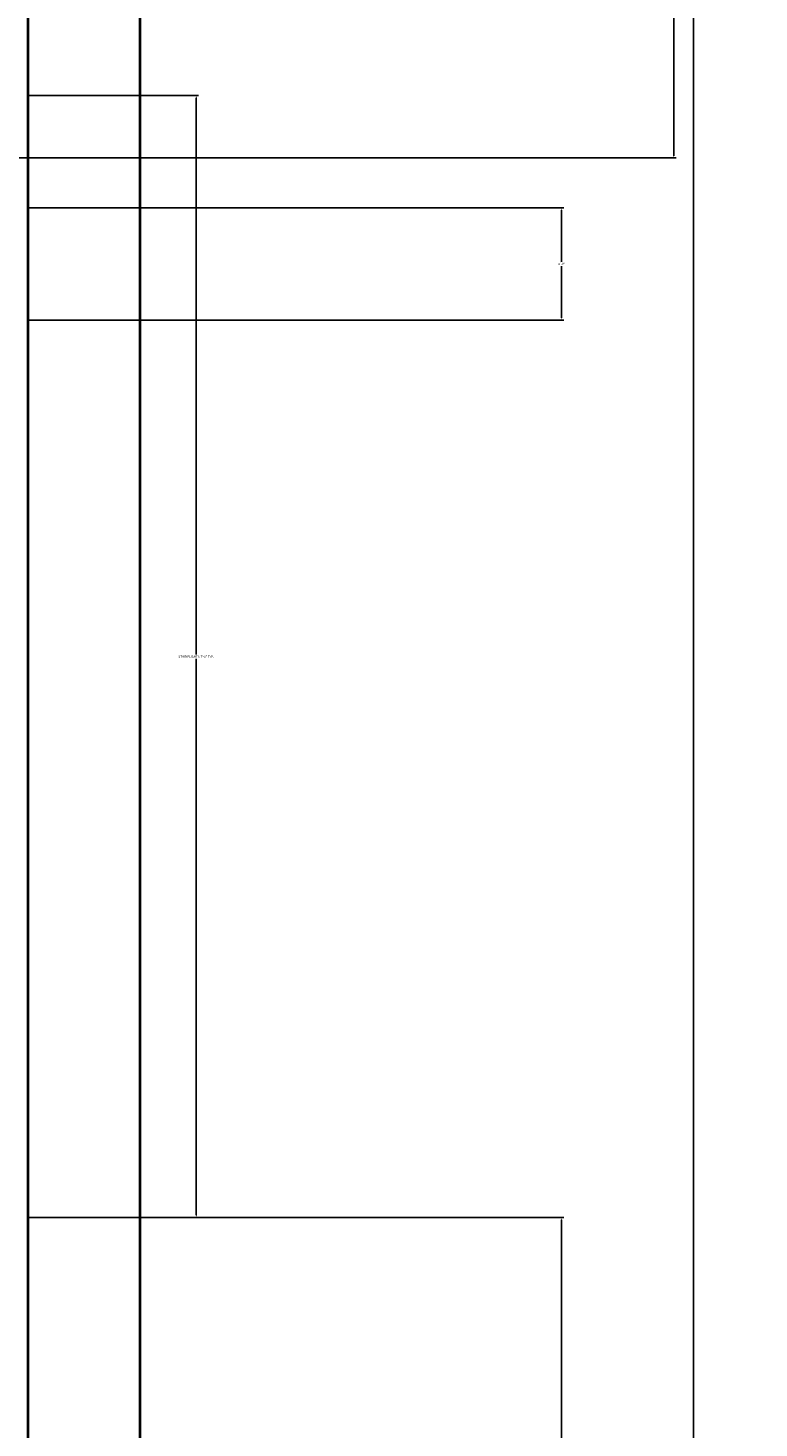
# Model space of a CAD drawing. Units: inches. Extents: x 182 to 1022, y -617 to 111.
# Tile 26 of 33: x 963 to 1022, y -507 to -395. Entities that reach past the tile are written whole.
import ezdxf

# ---------------------------------------------------------------- set-up
doc = ezdxf.new("R2010")
doc.units = ezdxf.units.IN
doc.header["$MEASUREMENT"] = 0
doc.layers.add('A-ANNO-DIMS', color=2, linetype='Continuous', lineweight=18)
doc.layers.add('wall', color=1, linetype='Continuous', lineweight=40)
doc.styles.get("Standard").update_dxf_attribs({"font": 'arial.ttf'})
doc.dimstyles.get("Standard").update_dxf_attribs({"dimtxt": 0.18, "dimasz": 0.18, "dimexe": 0.18, "dimexo": 0.0625, "dimgap": 0.09, "dimtad": 0, "dimtih": 1, "dimtoh": 1, "dimdec": 1, "dimzin": 0, "dimdsep": 46, "dimlunit": 4, "dimtxsty": 'Standard', "dimcen": 0.09, "dimadec": 0, "dimazin": 0, "dimtfac": 1, "dimtdec": 1, "dimtofl": 0, "dimtmove": 0, "dimatfit": 3, "dimfxl": 1, "dimtolj": 1, "dimtzin": 0, "dimarcsym": 0})

# ---------------------------------------------------------------- blocks, each defined once
blk = doc.blocks.new('_ArchTick')
at = {"color": 0, "linetype": 'ByBlock', "const_width": 0.15}
blk.add_lwpolyline([(-0.5, -0.5), (0.5, 0.5)], dxfattribs=at)
blk = doc.blocks.new('*D8')
at = {"layer": 'A-ANNO-DIMS', "color": 0, "lineweight": -2, "transparency": 16777216}
for p, q in [((1016.69, -0.37), (1016.69, -260.42)), ((1016.69, -540.37), (1016.69, -280.32))]:
    blk.add_line(p, q, dxfattribs=at)
at = {"layer": 'Defpoints', "color": 0, "transparency": 16777216}
for p in [(972.3, -0.37), (972.3, -540.37), (1016.69, -540.37)]:
    blk.add_point(p, dxfattribs=at)
at = {"layer": 'A-ANNO-DIMS', "color": 0, "lineweight": -2, "transparency": 16777216, "xscale": 8, "yscale": 8, "zscale": 8}
for p, rotation in [((1016.69, -0.37), 90), ((1016.69, -540.37), 270)]:
    blk.add_blockref('_ArchTick', p, dxfattribs=dict(at, rotation=rotation))
at = {"layer": 'A-ANNO-DIMS', "color": 0, "transparency": 16777216, "insert": (1016.69, -270.37), "char_height": 8, "attachment_point": 5, "rotation": 90}
blk.add_mtext("\\A1;45'", dxfattribs=at)
blk = doc.blocks.new('*D28')
at = {"layer": 'A-ANNO-DIMS', "color": 0, "lineweight": -2, "transparency": 16777216}
for p, q in [((963.37, -400.37), (976.98, -400.37)), ((976.8, -400.55), (976.8, -445.19)), ((976.8, -490.19), (976.8, -445.56)), ((963.37, -490.37), (976.98, -490.37))]:
    blk.add_line(p, q, dxfattribs=at)
at = {"layer": 'A-ANNO-DIMS', "color": 0, "transparency": 16777216}
for points in [[(976.77, -400.55), (976.83, -400.55), (976.8, -400.37)], [(976.77, -490.19), (976.83, -490.19), (976.8, -490.37)]]:
    blk.add_solid(points, dxfattribs=at)
at = {"layer": 'Defpoints', "color": 0, "transparency": 16777216}
for p in [(963.3, -400.37), (976.8, -400.37), (963.3, -490.37)]:
    blk.add_point(p, dxfattribs=at)
at = {"layer": 'A-ANNO-DIMS', "color": 0, "transparency": 16777216, "insert": (976.8, -445.37), "char_height": 0.18, "attachment_point": 5}
blk.add_mtext('\\A1;STAIR FLIGHTS 7\'-6" TYP.', dxfattribs=at)
blk = doc.blocks.new('*D39')
at = {"layer": 'A-ANNO-DIMS', "color": 0, "lineweight": -2, "transparency": 16777216}
for p, q in [((238.4, -288.54), (1015.28, -288.54)), ((1015.1, -288.72), (1015.1, -346.77)), ((1015.1, -405.19), (1015.1, -347.14)), ((238.43, -405.37), (1015.28, -405.37))]:
    blk.add_line(p, q, dxfattribs=at)
at = {"layer": 'A-ANNO-DIMS', "color": 0, "transparency": 16777216}
for points in [[(1015.07, -288.72), (1015.13, -288.72), (1015.1, -288.54)], [(1015.07, -405.19), (1015.13, -405.19), (1015.1, -405.37)]]:
    blk.add_solid(points, dxfattribs=at)
at = {"layer": 'Defpoints', "color": 0, "transparency": 16777216}
for p in [(238.34, -288.54), (1015.1, -288.54), (238.36, -405.37)]:
    blk.add_point(p, dxfattribs=at)
at = {"layer": 'A-ANNO-DIMS', "color": 0, "transparency": 16777216, "insert": (1015.1, -346.96), "char_height": 0.18, "attachment_point": 5}
blk.add_mtext('\\A1;9\'-9"', dxfattribs=at)
blk = doc.blocks.new('*D45')
at = {"layer": 'A-ANNO-DIMS', "color": 0, "lineweight": -2, "transparency": 16777216}
for p, q in [((963.37, -490.37), (1006.28, -490.37)), ((1006.1, -490.55), (1006.1, -510.69)), ((1006.1, -531.19), (1006.1, -511.06)), ((963.37, -531.37), (1006.28, -531.37))]:
    blk.add_line(p, q, dxfattribs=at)
at = {"layer": 'A-ANNO-DIMS', "color": 0, "transparency": 16777216}
for points in [[(1006.07, -490.55), (1006.13, -490.55), (1006.1, -490.37)], [(1006.07, -531.19), (1006.13, -531.19), (1006.1, -531.37)]]:
    blk.add_solid(points, dxfattribs=at)
at = {"layer": 'Defpoints', "color": 0, "transparency": 16777216}
for p in [(963.3, -490.37), (963.3, -531.37), (1006.1, -531.37)]:
    blk.add_point(p, dxfattribs=at)
at = {"layer": 'A-ANNO-DIMS', "color": 0, "transparency": 16777216, "insert": (1006.1, -510.87), "char_height": 0.18, "attachment_point": 5}
blk.add_mtext('\\A1;3\'-5"', dxfattribs=at)
blk = doc.blocks.new('*D46')
at = {"layer": 'A-ANNO-DIMS', "color": 0, "lineweight": -2, "transparency": 16777216}
for p, q in [((963.37, -409.37), (1006.28, -409.37)), ((1006.1, -409.55), (1006.1, -413.69)), ((1006.1, -418.19), (1006.1, -414.06)), ((963.37, -418.37), (1006.28, -418.37))]:
    blk.add_line(p, q, dxfattribs=at)
at = {"layer": 'A-ANNO-DIMS', "color": 0, "transparency": 16777216}
for points in [[(1006.07, -409.55), (1006.13, -409.55), (1006.1, -409.37)], [(1006.07, -418.19), (1006.13, -418.19), (1006.1, -418.37)]]:
    blk.add_solid(points, dxfattribs=at)
at = {"layer": 'Defpoints', "color": 0, "transparency": 16777216}
for p in [(963.3, -409.37), (963.3, -418.37), (1006.1, -418.37)]:
    blk.add_point(p, dxfattribs=at)
at = {"layer": 'A-ANNO-DIMS', "color": 0, "transparency": 16777216, "insert": (1006.1, -413.87), "char_height": 0.18, "attachment_point": 5}
blk.add_mtext('\\A1;0\'-9"', dxfattribs=at)

msp = doc.modelspace()

# ---------------------------------------------------------------- linework, layer by layer
at = {"layer": 'wall'}
for p, q in [((972.3, -540.37), (972.3, -0.37)), ((963.3, -322.87), (963.3, -531.37))]:
    msp.add_line(p, q, dxfattribs=at)

# ---------------------------------------------------------------- dimensions: what is measured, and where the dimension line sits
at = {"layer": 'A-ANNO-DIMS'}
for base, p1, p2, angle, override, picture, middle in [((1016.69, -540.37), (972.3, -0.37), (972.3, -540.37), 90, {"dimtxt": 8, "dimasz": 8, "dimgap": 3, "dimtih": 0, "dimblk1": 'ArchTick', "dimblk2": 'ArchTick', "dimsah": 1, "dimse1": 1, "dimse2": 1, "dimclrd": 0, "dimclre": 0, "dimclrt": 0}, '*D8', (1016.69, -270.37)), ((1015.1, -288.54), (238.36, -405.37), (238.34, -288.54), 90, {"dimdec": 1, "dimlfac": 1, "dimrnd": 0, "dimzin": 1, "dimdsep": 46, "dimlunit": 4, "dimfrac": 2}, '*D39', (1015.1, -346.96)), ((1006.1, -418.37), (963.3, -409.37), (963.3, -418.37), 270, {"dimdec": 1, "dimlfac": 1, "dimrnd": 0, "dimzin": 1, "dimdsep": 46, "dimlunit": 4, "dimfrac": 2}, '*D46', (1006.1, -413.87)), ((1006.1, -531.37), (963.3, -490.37), (963.3, -531.37), 270, {"dimdec": 1, "dimlfac": 1, "dimrnd": 0, "dimzin": 1, "dimdsep": 46, "dimlunit": 4, "dimfrac": 2}, '*D45', (1006.1, -510.87))]:
    dim = msp.add_linear_dim(base=base, p1=p1, p2=p2, angle=angle, dimstyle='Standard', override=override, dxfattribs=at)
    dim.commit()
    dim.dimension.update_dxf_attribs({"geometry": picture, "text_midpoint": middle})
dim = msp.add_linear_dim(base=(976.8, -400.37), p1=(963.3, -490.37), p2=(963.3, -400.37), angle=90, text='STAIR FLIGHTS <> TYP.', dimstyle='Standard', override={"dimdec": 1, "dimlfac": 1, "dimrnd": 0, "dimzin": 1, "dimdsep": 46, "dimlunit": 4, "dimfrac": 2}, dxfattribs=at)
dim.commit()
dim.dimension.update_dxf_attribs({"geometry": '*D28', "text_midpoint": (976.8, -445.37)})

doc.saveas('drawing.dxf')
